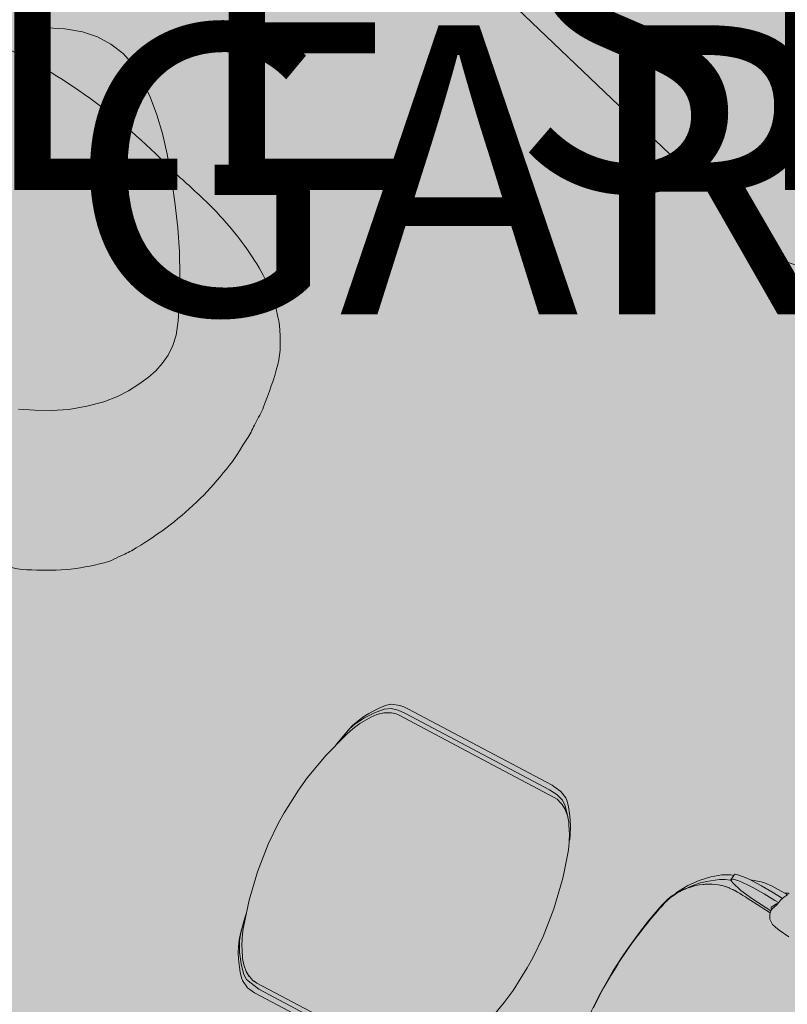
# Model space of a CAD drawing. Units: inches. Extents: x -466983 to 1020, y 324 to 318697.
# Tile 16 of 97: x 782.02 to 797.94, y 452.46 to 472.89. Entities that reach past the tile are written whole.
import ezdxf

# ---------------------------------------------------------------- set-up
doc = ezdxf.new("R2010")
doc.units = ezdxf.units.IN
doc.header["$MEASUREMENT"] = 0
for name, color, linetype, lineweight in [('A-ANNO-DIMS', 2, 'Continuous', 18), ('A-FLOR-PATT', 252, 'Continuous', 13), ('A-FURN', 8, 'Continuous', 18)]:
    doc.layers.add(name, color=color, linetype=linetype, lineweight=lineweight)
doc.layers.add('K-Hatch', color=7, linetype='Continuous')
doc.styles.get("Standard").update_dxf_attribs({"font": 'arial.ttf'})
doc.dimstyles.get("Standard").update_dxf_attribs({"dimtxt": 6, "dimasz": 4, "dimexe": 3, "dimexo": 3, "dimgap": 0.09, "dimtad": 0, "dimtih": 1, "dimtoh": 1, "dimdec": 1, "dimzin": 0, "dimdsep": 46, "dimlunit": 3, "dimtxsty": 'Standard', "dimcen": 0.09, "dimadec": 0, "dimazin": 0, "dimtfac": 1, "dimtdec": 1, "dimtofl": 0, "dimtmove": 0, "dimatfit": 3, "dimfxl": 1, "dimtolj": 1, "dimtzin": 0, "dimarcsym": 0})

# ---------------------------------------------------------------- blocks, each defined once
blk = doc.blocks.new('CBV_08')
at = {"layer": 'K-Hatch'}
h = blk.add_hatch(color=256, dxfattribs=at)
h.dxf.hatch_style = 1
h.set_gradient(color1=(254, 240, 205), color2=(128, 128, 128), name='INVSPHERICAL')
edge = h.paths.add_edge_path()
edge.add_line((-64.8, 606.5), (-20.8, 613.5))
edge.add_line((-20.8, 613.5), (24.3, 618.7))
edge.add_line((24.3, 618.7), (72.9, 622.4))
edge.add_line((72.9, 622.4), (121.2, 624.4))
edge.add_line((121.2, 624.4), (138, 624.4))
edge.add_spline(control_points=[(138, 624.4), (115.4, 642), (92.5, 659.2), (69.5, 676.1)], knot_values=[4, 4, 4, 4, 4.295361, 4.295361, 4.295361, 4.295361], degree=3, periodic=0)
edge.add_spline(control_points=[(69.5, 676.1), (30.7, 704.6), (-11, 728.2), (-55.3, 747.2)], knot_values=[3, 3, 3, 3, 4, 4, 4, 4], degree=3, periodic=0)
edge.add_spline(control_points=[(-55.3, 747.2), (-74.8, 755.6), (-96, 763.3), (-117, 767)], knot_values=[2, 2, 2, 2, 3, 3, 3, 3], degree=3, periodic=0)
edge.add_spline(control_points=[(-117, 767), (-129.2, 769.1), (-142.6, 773.4), (-154.9, 773.6)], knot_values=[1, 1, 1, 1, 2, 2, 2, 2], degree=3, periodic=0)
edge.add_spline(control_points=[(-154.9, 773.6), (-167.5, 773.8), (-180, 774.1), (-192.6, 774.3)], knot_values=[0, 0, 0, 0, 1, 1, 1, 1], degree=3, periodic=0)
edge.add_spline(control_points=[(-192.6, 774.3), (-216.8, 770.8), (-242.2, 768.1), (-264.6, 757.4)], knot_values=[36, 36, 36, 36, 37, 37, 37, 37], degree=3, periodic=0)
edge.add_spline(control_points=[(-264.6, 757.4), (-290.4, 745.1), (-313.9, 731.3), (-338.2, 716.3)], knot_values=[35, 35, 35, 35, 36, 36, 36, 36], degree=3, periodic=0)
edge.add_spline(control_points=[(-338.2, 716.3), (-348, 710.3), (-356.8, 702.3), (-365.9, 695.4)], knot_values=[34, 34, 34, 34, 35, 35, 35, 35], degree=3, periodic=0)
edge.add_spline(control_points=[(-365.9, 695.4), (-373.7, 689.5), (-381.9, 684), (-389, 677.3)], knot_values=[33, 33, 33, 33, 34, 34, 34, 34], degree=3, periodic=0)
edge.add_spline(control_points=[(-389, 677.3), (-406.7, 660.6), (-425.2, 644.6), (-441, 625.9)], knot_values=[32, 32, 32, 32, 33, 33, 33, 33], degree=3, periodic=0)
edge.add_spline(control_points=[(-441, 625.9), (-457.4, 606.6), (-473.1, 588.1), (-486.9, 566.8)], knot_values=[31, 31, 31, 31, 32, 32, 32, 32], degree=3, periodic=0)
edge.add_spline(control_points=[(-486.9, 566.8), (-500.9, 545.3), (-513.6, 524.6), (-525.3, 501.8)], knot_values=[30, 30, 30, 30, 31, 31, 31, 31], degree=3, periodic=0)
edge.add_spline(control_points=[(-525.3, 501.8), (-537.3, 478.5), (-547, 455.6), (-556.5, 431.1)], knot_values=[29, 29, 29, 29, 30, 30, 30, 30], degree=3, periodic=0)
edge.add_spline(control_points=[(-556.5, 431.1), (-560.1, 422), (-562.6, 413.9), (-564.7, 404.4)], knot_values=[28, 28, 28, 28, 29, 29, 29, 29], degree=3, periodic=0)
edge.add_spline(control_points=[(-564.7, 404.4), (-567.4, 392.4), (-572.8, 378.6), (-573.3, 366.3)], knot_values=[27, 27, 27, 27, 28, 28, 28, 28], degree=3, periodic=0)
edge.add_spline(control_points=[(-573.3, 366.3), (-574.1, 341.5), (-575.3, 317.8), (-572.6, 293.2)], knot_values=[26, 26, 26, 26, 27, 27, 27, 27], degree=3, periodic=0)
edge.add_spline(control_points=[(-572.6, 293.2), (-569.8, 268.3), (-564.7, 244.8), (-559.2, 220.4)], knot_values=[25, 25, 25, 25, 26, 26, 26, 26], degree=3, periodic=0)
edge.add_spline(control_points=[(-559.2, 220.4), (-554.1, 197.5), (-542.3, 175), (-531.2, 154.5)], knot_values=[24, 24, 24, 24, 25, 25, 25, 25], degree=3, periodic=0)
edge.add_spline(control_points=[(-531.2, 154.5), (-519.4, 132.5), (-505, 113.3), (-490.3, 93.1)], knot_values=[23, 23, 23, 23, 24, 24, 24, 24], degree=3, periodic=0)
edge.add_spline(control_points=[(-490.3, 93.1), (-483.4, 83.5), (-474, 75.1), (-466, 66.4)], knot_values=[22, 22, 22, 22, 23, 23, 23, 23], degree=3, periodic=0)
edge.add_spline(control_points=[(-466, 66.4), (-459.7, 59.5), (-453.6, 52.4), (-446.7, 46)], knot_values=[21, 21, 21, 21, 22, 22, 22, 22], degree=3, periodic=0)
edge.add_spline(control_points=[(-446.7, 46), (-428.9, 29.8), (-411.7, 12.8), (-392.8, -2.2)], knot_values=[20, 20, 20, 20, 21, 21, 21, 21], degree=3, periodic=0)
edge.add_spline(control_points=[(-392.8, -2.2), (-354.9, -32.3), (-316.7, -63.5), (-274.7, -87.8)], knot_values=[19, 19, 19, 19, 20, 20, 20, 20], degree=3, periodic=0)
edge.add_spline(control_points=[(-274.7, -87.8), (-235, -110.9), (-195.1, -133.6), (-153.3, -152.9)], knot_values=[18.058389, 18.058389, 18.058389, 18.058389, 19, 19, 19, 19], degree=3, periodic=0)
edge.add_arc((49.9, -261.3), 230.3, 65.0387, 151.9024, ccw=False)
edge.add_arc((-129.3, -568), 584.8, 31.4853, 61.8022, ccw=False)
edge.add_spline(control_points=[(369.5, -262.5), (382.1, -256.3), (394.4, -248.9), (404.8, -240.3)], knot_values=[14, 14, 14, 14, 14.639139, 14.639139, 14.639139, 14.639139], degree=3, periodic=0)
edge.add_spline(control_points=[(404.8, -240.3), (441.3, -209.9), (479.6, -177), (505.1, -136.3)], knot_values=[13, 13, 13, 13, 14, 14, 14, 14], degree=3, periodic=0)
edge.add_spline(control_points=[(505.1, -136.3), (530.8, -95.3), (553.2, -52.4), (563.4, -4.8)], knot_values=[12, 12, 12, 12, 13, 13, 13, 13], degree=3, periodic=0)
edge.add_spline(control_points=[(563.4, -4.8), (565.9, 6.8), (569.9, 18.9), (570.9, 30.6)], knot_values=[11, 11, 11, 11, 12, 12, 12, 12], degree=3, periodic=0)
edge.add_spline(control_points=[(570.9, 30.6), (572, 44.6), (573.1, 58.6), (574.2, 72.5)], knot_values=[10, 10, 10, 10, 11, 11, 11, 11], degree=3, periodic=0)
edge.add_spline(control_points=[(574.2, 72.5), (575.1, 84.1), (571.6, 97.4), (570.3, 109)], knot_values=[9, 9, 9, 9, 10, 10, 10, 10], degree=3, periodic=0)
edge.add_spline(control_points=[(570.3, 109), (569.1, 120.8), (562.9, 133.2), (559.3, 144.5)], knot_values=[8, 8, 8, 8, 9, 9, 9, 9], degree=3, periodic=0)
edge.add_spline(control_points=[(559.3, 144.5), (552.8, 164.6), (542, 184.7), (531.4, 203)], knot_values=[7, 7, 7, 7, 8, 8, 8, 8], degree=3, periodic=0)
edge.add_spline(control_points=[(531.4, 203), (517.9, 226.2), (504.2, 248.2), (488.9, 270.1)], knot_values=[6, 6, 6, 6, 7, 7, 7, 7], degree=3, periodic=0)
edge.add_spline(control_points=[(488.9, 270.1), (469.9, 297.6), (449.2, 323.8), (427.6, 349.1)], knot_values=[5.661323, 5.661323, 5.661323, 5.661323, 6, 6, 6, 6], degree=3, periodic=0)
edge.add_line((427.6, 349.1), (424, 340.6))
edge.add_line((424, 340.6), (412.8, 320.4))
edge.add_line((412.8, 320.4), (399.8, 302.2))
edge.add_line((399.8, 302.2), (384.1, 283.9))
edge.add_line((384.1, 283.9), (364.2, 265.4))
edge.add_line((364.2, 265.4), (338.9, 246.4))
edge.add_line((338.9, 246.4), (310.9, 228.8))
edge.add_line((310.9, 228.8), (283, 214))
edge.add_line((283, 214), (254.8, 200.7))
edge.add_line((254.8, 200.7), (225.6, 187.8))
edge.add_line((225.6, 187.8), (191.9, 174.7))
edge.add_line((191.9, 174.7), (149.8, 160.6))
edge.add_line((149.8, 160.6), (105.2, 147.1))
edge.add_line((105.2, 147.1), (63.8, 135.5))
edge.add_line((63.8, 135.5), (25.5, 126.4))
edge.add_line((25.5, 126.4), (-10.1, 120.3))
edge.add_line((-10.1, 120.3), (-42.7, 117))
edge.add_line((-42.7, 117), (-72.3, 116.4))
edge.add_line((-72.3, 116.4), (-101, 119.4))
edge.add_line((-101, 119.4), (-131.2, 126.4))
edge.add_line((-131.2, 126.4), (-161, 137.6))
edge.add_line((-161, 137.6), (-188.5, 153.1))
edge.add_line((-188.5, 153.1), (-212.6, 173.8))
edge.add_line((-212.6, 173.8), (-232.4, 200.6))
edge.add_line((-232.4, 200.6), (-247.5, 230.4))
edge.add_line((-247.5, 230.4), (-258, 260.2))
edge.add_line((-258, 260.2), (-265.5, 290.4))
edge.add_line((-265.5, 290.4), (-271.7, 321.1))
edge.add_line((-271.7, 321.1), (-275.7, 353.5))
edge.add_line((-275.7, 353.5), (-276.1, 388.5))
edge.add_line((-276.1, 388.5), (-273.5, 421.6))
edge.add_line((-273.5, 421.6), (-268.6, 448.2))
edge.add_line((-268.6, 448.2), (-261.6, 470.9))
edge.add_line((-261.6, 470.9), (-253.2, 492.6))
edge.add_line((-253.2, 492.6), (-243.7, 512.2))
edge.add_line((-243.7, 512.2), (-233.7, 528.6))
edge.add_line((-233.7, 528.6), (-222.4, 543.2))
edge.add_line((-222.4, 543.2), (-208.8, 557))
edge.add_line((-208.8, 557), (-193, 569.1))
edge.add_line((-193, 569.1), (-174.9, 578.6))
edge.add_line((-174.9, 578.6), (-149, 587.3))
edge.add_line((-149, 587.3), (-109.9, 597.2))
edge.add_line((-109.9, 597.2), (-64.8, 606.5))
edge = h.paths.add_edge_path()
edge.add_spline(control_points=[(370.8, -764.2), (495.7, -715.3), (556.2, -553.3), (490.4, -435.8)], knot_values=[8, 8, 8, 8, 9, 9, 9, 9], degree=3, periodic=0)
edge.add_spline(control_points=[(490.4, -435.8), (456.6, -375.3), (415.1, -316.6), (369.5, -262.5)], knot_values=[7.311196, 7.311196, 7.311196, 7.311196, 8, 8, 8, 8], degree=3, periodic=0)
edge.add_spline(control_points=[(369.5, -262.5), (362.3, -266), (355, -269.1), (347.9, -271.7)], knot_values=[14.639139, 14.639139, 14.639139, 14.639139, 15, 15, 15, 15], degree=3, periodic=0)
edge.add_spline(control_points=[(347.9, -271.7), (326, -279.9), (303.4, -287.9), (279.6, -286.9)], knot_values=[15, 15, 15, 15, 16, 16, 16, 16], degree=3, periodic=0)
edge.add_spline(control_points=[(279.6, -286.9), (229.3, -284.8), (181, -274.1), (132.3, -261.7)], knot_values=[16, 16, 16, 16, 17, 17, 17, 17], degree=3, periodic=0)
edge.add_spline(control_points=[(132.3, -261.7), (36, -237.2), (-55, -196.9), (-145.5, -156.4)], knot_values=[17, 17, 17, 17, 18, 18, 18, 18], degree=3, periodic=0)
edge.add_spline(control_points=[(-145.5, -156.4), (-148.1, -155.2), (-150.7, -154.1), (-153.3, -152.9)], knot_values=[18, 18, 18, 18, 18.058389, 18.058389, 18.058389, 18.058389], degree=3, periodic=0)
edge.add_spline(control_points=[(-274.7, -87.8), (-235, -110.9), (-195.1, -133.6), (-153.3, -152.9)], knot_values=[18.058389, 18.058389, 18.058389, 18.058389, 19, 19, 19, 19], degree=3, periodic=0)
edge.add_spline(control_points=[(-153.3, -152.9), (-166, -171.6), (-175.5, -191.9), (-179.2, -212.7)], knot_values=[4, 4, 4, 4, 4.452929, 4.452929, 4.452929, 4.452929], degree=3, periodic=0)
edge.add_spline(control_points=[(-179.2, -212.7), (-197.4, -316.3), (-177.2, -425), (-133.8, -520.2)], knot_values=[3, 3, 3, 3, 4, 4, 4, 4], degree=3, periodic=0)
edge.add_spline(control_points=[(-133.8, -520.2), (-113.8, -564.2), (-89.7, -609.8), (-55.6, -644.7)], knot_values=[2, 2, 2, 2, 3, 3, 3, 3], degree=3, periodic=0)
edge.add_spline(control_points=[(-55.6, -644.7), (-21, -680), (24.1, -705.5), (69.8, -723.3)], knot_values=[1, 1, 1, 1, 2, 2, 2, 2], degree=3, periodic=0)
edge.add_spline(control_points=[(69.8, -723.3), (165.7, -760.7), (268.3, -790.7), (370.8, -764.2)], knot_values=[0, 0, 0, 0, 1, 1, 1, 1], degree=3, periodic=0)
h = blk.add_hatch(color=256, dxfattribs=at)
h.dxf.hatch_style = 1
h.set_gradient(color1=(237, 238, 153), color2=(128, 128, 128), name='INVSPHERICAL')
h.paths.add_polyline_path([(138, 624.4), (121.2, 624.4), (72.9, 622.4), (24.3, 618.7), (-20.8, 613.5), (-64.8, 606.5), (-109.9, 597.2), (-149, 587.3), (-174.9, 578.6), (-193, 569.1), (-208.8, 557), (-222.4, 543.2), (-233.7, 528.6), (-243.7, 512.2), (-253.2, 492.6), (-261.6, 470.9), (-268.6, 448.2), (-273.5, 421.6), (-276.1, 388.5), (-275.7, 353.5), (-271.7, 321.1), (-265.5, 290.4), (-258, 260.2), (-247.5, 230.4), (-232.4, 200.6), (-212.6, 173.8), (-188.5, 153.1), (-161, 137.6), (-131.2, 126.4), (-101, 119.4), (-72.3, 116.4), (-42.7, 117), (-10.1, 120.3), (25.5, 126.4), (63.8, 135.5), (105.2, 147.1), (149.8, 160.6), (191.9, 174.7), (225.6, 187.8), (254.8, 200.7), (283, 214), (310.9, 228.8), (338.9, 246.4), (364.2, 265.4), (384.1, 283.9), (399.8, 302.2), (412.8, 320.4), (424, 340.6), (427.6, 349.1, 0.092765)])
h.paths.add_polyline_path([(388.8, 558), (367.1, 577.3), (341.1, 593.1), (309.7, 604.8), (275.6, 613.2), (241.4, 619.1), (205.2, 622.8), (165.2, 624.5), (138, 624.4, -0.092765), (427.6, 349.1), (434.3, 364.7), (441.6, 390.8), (443.8, 416.8), (441.1, 445), (433.5, 477.6), (421.8, 509.5), (406.9, 535.9)])
edge = h.paths.add_edge_path()
edge.add_arc((49.9, -261.3), 230.3, 65.0387, 151.9024)
edge.add_spline(control_points=[(-153.3, -152.9), (-150.7, -154.1), (-148.1, -155.2), (-145.5, -156.4)], knot_values=[18, 18, 18, 18, 18.058389, 18.058389, 18.058389, 18.058389], degree=3, periodic=0)
edge.add_spline(control_points=[(-145.5, -156.4), (-55, -196.9), (36, -237.2), (132.3, -261.7)], knot_values=[17, 17, 17, 17, 18, 18, 18, 18], degree=3, periodic=0)
edge.add_spline(control_points=[(132.3, -261.7), (181, -274.1), (229.3, -284.8), (279.6, -286.9)], knot_values=[16, 16, 16, 16, 17, 17, 17, 17], degree=3, periodic=0)
edge.add_spline(control_points=[(279.6, -286.9), (303.4, -287.9), (326, -279.9), (347.9, -271.7)], knot_values=[15, 15, 15, 15, 16, 16, 16, 16], degree=3, periodic=0)
edge.add_spline(control_points=[(347.9, -271.7), (355, -269.1), (362.3, -266), (369.5, -262.5)], knot_values=[14.639139, 14.639139, 14.639139, 14.639139, 15, 15, 15, 15], degree=3, periodic=0)
edge.add_arc((-129.3, -568), 584.8, 31.4853, 61.8022)
edge = h.paths.add_edge_path()
edge.add_spline(control_points=[(490.4, -435.8), (456.6, -375.3), (415.1, -316.6), (369.5, -262.5)], knot_values=[7.311196, 7.311196, 7.311196, 7.311196, 8, 8, 8, 8], degree=3, periodic=0)
edge.add_spline(control_points=[(369.5, -262.5), (362.3, -266), (355, -269.1), (347.9, -271.7)], knot_values=[14.639139, 14.639139, 14.639139, 14.639139, 15, 15, 15, 15], degree=3, periodic=0)
edge.add_spline(control_points=[(347.9, -271.7), (326, -279.9), (303.4, -287.9), (279.6, -286.9)], knot_values=[15, 15, 15, 15, 16, 16, 16, 16], degree=3, periodic=0)
edge.add_spline(control_points=[(279.6, -286.9), (229.3, -284.8), (181, -274.1), (132.3, -261.7)], knot_values=[16, 16, 16, 16, 17, 17, 17, 17], degree=3, periodic=0)
edge.add_spline(control_points=[(132.3, -261.7), (36, -237.2), (-55, -196.9), (-145.5, -156.4)], knot_values=[17, 17, 17, 17, 18, 18, 18, 18], degree=3, periodic=0)
edge.add_spline(control_points=[(-145.5, -156.4), (-148.1, -155.2), (-150.7, -154.1), (-153.3, -152.9)], knot_values=[18, 18, 18, 18, 18.058389, 18.058389, 18.058389, 18.058389], degree=3, periodic=0)
edge.add_spline(control_points=[(-274.7, -87.8), (-235, -110.9), (-195.1, -133.6), (-153.3, -152.9)], knot_values=[18.058389, 18.058389, 18.058389, 18.058389, 19, 19, 19, 19], degree=3, periodic=0)
edge.add_spline(control_points=[(-153.3, -152.9), (-166, -171.6), (-175.5, -191.9), (-179.2, -212.7)], knot_values=[4, 4, 4, 4, 4.452929, 4.452929, 4.452929, 4.452929], degree=3, periodic=0)
edge.add_spline(control_points=[(-179.2, -212.7), (-197.4, -316.3), (-177.2, -425), (-133.8, -520.2)], knot_values=[3, 3, 3, 3, 4, 4, 4, 4], degree=3, periodic=0)
edge.add_spline(control_points=[(-133.8, -520.2), (-113.8, -564.2), (-89.7, -609.8), (-55.6, -644.7)], knot_values=[2, 2, 2, 2, 3, 3, 3, 3], degree=3, periodic=0)
edge.add_spline(control_points=[(-55.6, -644.7), (-21, -680), (24.1, -705.5), (69.8, -723.3)], knot_values=[1, 1, 1, 1, 2, 2, 2, 2], degree=3, periodic=0)
edge.add_spline(control_points=[(69.8, -723.3), (165.7, -760.7), (268.3, -790.7), (370.8, -764.2)], knot_values=[0, 0, 0, 0, 1, 1, 1, 1], degree=3, periodic=0)
edge.add_spline(control_points=[(370.8, -764.2), (495.7, -715.3), (556.2, -553.3), (490.4, -435.8)], knot_values=[8, 8, 8, 8, 9, 9, 9, 9], degree=3, periodic=0)
for points in [[(24.3, 618.7), (-20.8, 613.5)], [(72.9, 622.4), (24.3, 618.7)], [(121.2, 624.4), (72.9, 622.4)], [(121.2, 624.4), (72.9, 622.4)], [(165.2, 624.5), (121.2, 624.4)], [(205.2, 622.8), (165.2, 624.5)], [(241.4, 619.1), (205.2, 622.8)], [(275.6, 613.2), (241.4, 619.1)], [(-109.9, 597.2), (-149, 587.3)], [(-64.8, 606.5), (-109.9, 597.2)], [(-20.8, 613.5), (-64.8, 606.5)], [(309.7, 604.8), (275.6, 613.2)], [(341.1, 593.1), (309.7, 604.8)], [(-174.9, 578.6), (-193, 569.1)], [(-149, 587.3), (-174.9, 578.6)], [(367.1, 577.3), (341.1, 593.1)], [(388.8, 558), (367.1, 577.3)], [(-193, 569.1), (-208.8, 557)], [(-222.4, 543.2), (-233.7, 528.6)], [(-208.8, 557), (-222.4, 543.2)], [(406.9, 535.9), (388.8, 558)], [(-233.7, 528.6), (-243.7, 512.2)], [(421.8, 509.5), (406.9, 535.9)], [(-243.7, 512.2), (-253.2, 492.6)], [(433.5, 477.6), (421.8, 509.5)], [(-253.2, 492.6), (-261.6, 470.9)], [(-261.6, 470.9), (-268.6, 448.2)], [(441.1, 445), (433.5, 477.6)], [(-268.6, 448.2), (-273.5, 421.6)], [(443.8, 416.8), (441.1, 445)], [(-273.5, 421.6), (-276.1, 388.5)], [(441.6, 390.8), (443.8, 416.8)], [(-276.1, 388.5), (-275.7, 353.5)], [(-275.7, 353.5), (-271.7, 321.1)], [(-271.7, 321.1), (-265.5, 290.4)], [(-265.5, 290.4), (-258, 260.2)]]:
    blk.add_lwpolyline(points)
at = {"ltscale": 150}
blk.add_arc((-452.8, -286.9), 1086.1, 35.8442, 57.0436, dxfattribs=at)
for points, knots in [([(427.6, 349.1), (449.2, 323.8), (469.9, 297.6), (488.9, 270.1), (504.2, 248.2), (517.9, 226.2), (531.4, 203), (542, 184.7), (552.8, 164.6), (559.3, 144.5), (562.9, 133.2), (569.1, 120.8), (570.3, 109), (571.6, 97.4), (575.1, 84.1), (574.2, 72.5), (573.1, 58.6), (572, 44.6), (570.9, 30.6), (569.9, 18.9), (565.9, 6.8), (563.4, -4.8), (553.2, -52.4), (530.8, -95.3), (505.1, -136.3), (479.6, -177), (441.3, -209.9), (404.8, -240.3), (388.6, -253.7), (367.6, -264.4), (347.9, -271.7), (326, -279.9), (303.4, -287.9), (279.6, -286.9), (229.3, -284.8), (181, -274.1), (132.3, -261.7), (36, -237.2), (-55, -196.9), (-145.5, -156.4), (-190.2, -136.4), (-232.5, -112.4), (-274.7, -87.8), (-316.7, -63.5), (-354.9, -32.3), (-392.8, -2.2), (-411.7, 12.8), (-428.9, 29.8), (-446.7, 46), (-453.6, 52.4), (-459.7, 59.5), (-466, 66.4), (-474, 75.1), (-483.4, 83.5), (-490.3, 93.1), (-505, 113.3), (-519.4, 132.5), (-531.2, 154.5), (-542.3, 175), (-554.1, 197.5), (-559.2, 220.4), (-564.7, 244.8), (-569.8, 268.3), (-572.6, 293.2), (-575.3, 317.8), (-574.1, 341.5), (-573.3, 366.3), (-572.8, 378.6), (-567.4, 392.4), (-564.7, 404.4), (-562.6, 413.9), (-560.1, 422), (-556.5, 431.1), (-547, 455.6), (-537.3, 478.5), (-525.3, 501.8), (-513.6, 524.6), (-500.9, 545.3), (-486.9, 566.8), (-473.1, 588.1), (-457.4, 606.6), (-441, 625.9), (-425.2, 644.6), (-406.7, 660.6), (-389, 677.3), (-381.9, 684), (-373.7, 689.5), (-365.9, 695.4), (-356.8, 702.3), (-348, 710.3), (-338.2, 716.3), (-313.9, 731.3), (-290.4, 745.1), (-264.6, 757.4), (-242.2, 768.1), (-216.8, 770.8), (-192.6, 774.3)], [5.661323, 5.661323, 5.661323, 5.661323, 6, 6, 6, 7, 7, 7, 8, 8, 8, 9, 9, 9, 10, 10, 10, 11, 11, 11, 12, 12, 12, 13, 13, 13, 14, 14, 14, 15, 15, 15, 16, 16, 16, 17, 17, 17, 18, 18, 18, 19, 19, 19, 20, 20, 20, 21, 21, 21, 22, 22, 22, 23, 23, 23, 24, 24, 24, 25, 25, 25, 26, 26, 26, 27, 27, 27, 28, 28, 28, 29, 29, 29, 30, 30, 30, 31, 31, 31, 32, 32, 32, 33, 33, 33, 34, 34, 34, 35, 35, 35, 36, 36, 36, 37, 37, 37, 37]), ([(-192.6, 774.3), (-180, 774.1), (-167.5, 773.8), (-154.9, 773.6), (-142.6, 773.4), (-129.2, 769.1), (-117, 767), (-96, 763.3), (-74.8, 755.6), (-55.3, 747.2), (-11, 728.2), (30.7, 704.6), (69.5, 676.1), (92.5, 659.2), (115.4, 642), (138, 624.4)], [0, 0, 0, 0, 1, 1, 1, 2, 2, 2, 3, 3, 3, 4, 4, 4, 4.295361, 4.295361, 4.295361, 4.295361])]:
    blk.add_open_spline(points, degree=3, knots=knots)
blk = doc.blocks.new('CBV_05')
at = {"layer": 'K-Hatch'}
h = blk.add_hatch(color=256, dxfattribs=at)
h.dxf.hatch_style = 1
h.paths.add_polyline_path([(614, 437), (1251.4, 62.5), (1198.3, -263.2), (564.8, -9.8), (344.4, -5.5), (343.7, -629.7, 0.159768), (369.9, -672.6), (1020.5, -1025.6, 0.317347), (1135.5, -1017.7), (1739.5, -492.7, 0.378101), (1761.2, -362.2), (1507.4, -70.4, -0.119239), (1492.6, -25.8), (1499.5, 665.1, 0.256804), (1446.2, 745.4), (822.7, 1028.7, 0.297137), (714, 1018.3), (625, 963.6), (549.5, 1037.1), (186.8, 587.5), (-1106.2, 397.7), (-1098.6, 311.5), (-1098.4, 310.2)])
h.paths.add_polyline_path([(344.4, -5.5), (-1216.9, 24.6), (-1212.3, 260), (-1718.1, 162.7, 0.51466), (-1765.1, 50), (-1478.1, -479.5, 0.244482), (-1398.8, -526.6), (323.6, -658.2, 0.453292), (343.1, -629.8, 0.006511), (343.7, -631.8)])
blk.add_lwpolyline([(1761.2, -362.2, -0.378101), (1739.5, -492.7), (1135.5, -1017.7, -0.317347), (1020.5, -1025.6), (369.9, -672.6, -0.159481), (343.2, -630.1, -0.449095), (323.6, -658.2), (-1398.8, -526.6, -0.244482), (-1478.1, -479.5), (-1765.1, 50, -0.51466), (-1718.1, 162.7), (-1212.3, 260), (-1211.5, 301.9), (-1098.4, 310.2), (-1106.2, 397.7), (186.8, 587.5), (549.5, 1037.1), (625, 963.6), (714, 1018.3, -0.297137), (822.7, 1028.7), (1446.2, 745.4, -0.256804), (1499.5, 665.1), (1492.6, -25.8, 0.119239), (1507.4, -70.4)], format="xyb", close=True)
blk.add_lwpolyline([(-1212.3, 260), (-1718.1, 162.7, 0.51466), (-1765.1, 50), (-1478.1, -479.5, 0.244482), (-1398.8, -526.6), (323.6, -658.2)], format="xyb")
blk = doc.blocks.new('CBV_11')
at = {"layer": 'K-Hatch'}
h = blk.add_hatch(color=256, dxfattribs=at)
h.dxf.hatch_style = 1
h.paths.add_polyline_path([(-178.4, 698.3), (-200.4, 717.9), (-207.1, 720), (-213, 721.7), (-231.8, 722.5), (-254.2, 721.5), (-275, 717.7), (-289.3, 712.5), (-316, 699.4), (-324.9, 694.8), (-295.8, 706.5), (-286.8, 709.3), (-277.1, 712.2), (-265.3, 715), (-258.1, 715.9), (-241.3, 718.1), (-228.8, 718), (-215.5, 715.7), (-208.8, 713.2), (-205.5, 711.6), (-203.9, 710.6), (-202.4, 709.7), (-195.4, 705.2), (-194.8, 704.5), (-190.4, 699.8), (-87.3, 570), (16.1, 440.3), (19.6, 435), (22.9, 426.4), (24.1, 422.9), (25.8, 412.3), (25.1, 398.9), (24.2, 394.5), (25.6, 399.8), (28.8, 418.8), (27.5, 432), (13.6, 457)])
h.paths.add_polyline_path([(-536, 213.1), (-639.3, 342.7), (-642.9, 348.1), (-646.2, 356.7), (-647.4, 360.2), (-649.1, 370.8), (-648.4, 384.2), (-645.7, 396.4), (-637.3, 419.1), (-631.8, 430), (-626.9, 438.8), (-622.1, 446.9), (-606.5, 469.3), (-631, 439.9), (-638.6, 427.4), (-646.5, 408.6), (-652.3, 388), (-655.6, 368.8), (-654.4, 355.7), (-649, 343.1), (-640.5, 330.7), (-448.6, 89.4), (-437.6, 77.7), (-424.8, 69.2), (-413.8, 65.9), (-392.4, 64.7), (-388.1, 65), (-394.5, 65), (-407.8, 67.4), (-417, 71.1), (-420.9, 73.4), (-427.9, 77.9), (-428.5, 78.6), (-432.9, 83.2)])
for points in [[(21.3, 463.1), (-173.2, 707.5), (-185, 718.7), (-200.1, 726), (-205.3, 726.9), (-216.4, 727.2), (-226.1, 726.9), (-241.2, 725.8), (-253.7, 723.9), (-264.9, 721.5), (-277.2, 717.9), (-288.3, 713.3), (-311.8, 701.8), (-324.9, 694.8), (-316, 699.4), (-289.3, 712.5), (-275, 717.7), (-254.2, 721.5), (-231.8, 722.5), (-213, 721.7), (-207.1, 720), (-200.4, 717.9), (-178.4, 698.3), (13.6, 457)], [(-87.3, 570), (-190.4, 699.8), (-194.8, 704.5), (-195.4, 705.2), (-202.4, 709.7), (-203.9, 710.6), (-208.8, 713.2), (-215.5, 715.7), (-228.8, 718), (-241.3, 718.1), (-258.1, 715.9), (-265.3, 715), (-277.1, 712.2), (-286.8, 709.3), (-295.8, 706.5), (-324.9, 694.8), (-347.4, 685.7), (-397.3, 660.4), (-444.8, 630.8), (-480.8, 604.2), (-497.4, 590.5), (-534.5, 556.2), (-554.4, 535.5), (-590.2, 492.6), (-603.5, 473.5), (-606.5, 469.3), (-622.1, 446.9), (-626.9, 438.8), (-631.8, 430), (-637.3, 419.1), (-645.7, 396.4), (-648.4, 384.2), (-649.1, 370.8), (-647.4, 360.2), (-646.2, 356.7), (-642.9, 348.1), (-639.3, 342.7), (-536, 213.1), (-432.9, 83.2), (-428.5, 78.6), (-427.9, 77.9), (-420.9, 73.4), (-417, 71.1), (-407.8, 67.4), (-394.5, 65), (-388.1, 65), (-382, 64.9), (-376.6, 65.6), (-368.3, 66.6), (-367.7, 66.7), (-359.3, 67.5), (-346.5, 70.4), (-345.9, 70.6), (-336.1, 73.3), (-327.3, 76.2), (-282.4, 94.4), (-275.6, 97.1), (-225.7, 122.4), (-178.3, 151.9), (-142.2, 178.6), (-125.6, 192.2), (-88.5, 226.6), (-68.7, 247.3), (-32.9, 290.2)], [(-203.9, 710.6), (-205.5, 711.6), (-208.8, 713.2)], [(-346.5, 70.4), (-349.3, 69.2), (-356.8, 67), (-372.9, 63.3), (-385.5, 61.5), (-398.1, 60.5), (-410.3, 60.2), (-421.5, 60.6), (-428.5, 61.9), (-441.8, 68.9), (-453.7, 80.2), (-456.3, 83.2), (-648.2, 324.6), (-653.1, 331.3), (-657.2, 338.3), (-662.3, 353.4), (-662.3, 363.4), (-659.9, 375.1), (-656.8, 387), (-652.8, 399), (-648.1, 410.9), (-642.7, 422.1), (-636.8, 432.3), (-630.4, 441.2), (-607, 469.6), (-603.5, 473.5)], [(-606.5, 469.3), (-631, 439.9), (-638.6, 427.4), (-646.5, 408.6), (-652.3, 388), (-655.6, 368.8), (-654.4, 355.7), (-649, 343.1), (-640.5, 330.7), (-448.6, 89.4), (-437.6, 77.7), (-424.8, 69.2), (-413.8, 65.9), (-392.4, 64.7), (-388.1, 65)], [(-50.1, 67.5), (-23.5, 87.9), (-9.9, 97.6), (3.8, 107.1), (17.8, 116.4), (31.9, 125.3), (60.6, 142.4), (89.9, 158.3), (119.5, 173.3), (135, 179.9), (142.8, 182.8), (151, 184.8), (159.6, 185.9), (175.9, 186.9), (181, 186.7)], [(-28.5, 83.3), (-36.4, 77.2), (-38.8, 75.4), (-45.1, 70.6), (-49.7, 67), (-54.2, 63.4), (-56, 61.9), (-62.5, 56.6), (-75.5, 45.6), (-77.3, 44), (-77.4, 44)], [(-217.7, -216.8), (-218.7, -214.8), (-221.6, -206), (-223.5, -195.1), (-224.4, -170.3), (-223.2, -156.5), (-220.9, -142.4), (-219, -134.5), (-218.9, -134.4), (-218.9, -134.2), (-217.3, -125.9), (-215.2, -117.7), (-212.7, -109.9), (-212.1, -108.4), (-207.7, -98.2), (-203.6, -90.8), (-196.4, -80.6), (-191.3, -74), (-180.9, -61.1), (-170.2, -48.3), (-159.1, -35.9), (-159.1, -35.8), (-148, -23.5), (-124.9, 0.7), (-113, 12.4), (-100.8, 23.9), (-88.5, 35.1), (-75.9, 46.2), (-63.1, 57), (-50.1, 67.5)], [(-214.7, -118), (-214.6, -117.8), (-212.4, -111.4), (-210.9, -107.7), (-210.4, -106.5), (-210.1, -105.7), (-209.4, -104.2), (-209, -103.5), (-206, -97.3), (-205.1, -95.8), (-204.7, -95), (-203.9, -93.8), (-203.5, -93.2), (-202.6, -91.5), (-202, -90.5), (-200.3, -88.1), (-199.3, -86.6), (-198.2, -84.9), (-198, -84.7), (-197.9, -84.5), (-192.8, -77.9), (-190.9, -75.4), (-190.5, -74.9), (-189.8, -74), (-186.5, -69.8), (-173.8, -54.2), (-170.7, -50.6), (-169.2, -48.8), (-167, -46.3), (-160.8, -39.1), (-147.5, -24.2), (-147.4, -24.1), (-147.3, -24), (-146.9, -23.6), (-146.4, -23.1), (-134, -9.8), (-127, -2.7), (-124.7, -0.3), (-124.4, -0.1), (-124.2, 0.2), (-123.2, 1.2), (-120.2, 4.2), (-106.2, 17.9), (-102.9, 20.9), (-101.4, 22.4), (-98.9, 24.6), (-91.9, 31.1), (-77.7, 43.7), (-77.6, 43.8), (-77.4, 44)], [(-212.1, -108.4), (-213.8, -111.2), (-223, -134.4), (-228.6, -157.2), (-231.3, -180.4), (-231, -201.3), (-228.1, -217.6), (-225.8, -223.3), (-226.1, -223.6), (-227.6, -226.1), (-224.9, -232.9), (-218.3, -243.6), (-212.6, -251.5), (-209.6, -255.8), (-197.1, -271.4), (-182.6, -288.2), (-173.4, -298.4), (-166.3, -306.1)], [(-143.8, -278.1), (-149.7, -271.9), (-151.2, -270.2), (-153.6, -267.6), (-153.7, -267.6), (-158.2, -262.7), (-179.1, -240.4), (-181.9, -237.4), (-184, -235.2), (-185.8, -233.2), (-188.4, -230.4), (-188.8, -230), (-189.2, -229.5), (-191, -227.5), (-192.6, -225.7), (-192.9, -225.2), (-193.3, -224.8), (-194.6, -223.3), (-196.5, -221), (-197, -220.3), (-197.5, -219.7), (-198.5, -218.3), (-200, -216.4), (-200.2, -216.2), (-201.3, -214.6), (-201.4, -214.5), (-203.2, -212), (-203.8, -211.2), (-204.4, -210.2), (-205.3, -208.8), (-206.1, -207.6), (-206.2, -207.4), (-206.3, -207.3), (-206.4, -207), (-206.6, -206.8), (-207.1, -206), (-207.5, -205.3), (-207.5, -205.2), (-207.6, -205.1), (-207.6, -205), (-208.1, -204.2), (-208.2, -204), (-208.3, -203.8), (-208.4, -203.7), (-208.7, -203.2), (-209.4, -202), (-209.4, -201.9), (-209.6, -201.7), (-210.3, -200.2), (-211.3, -198.2), (-211.5, -197.7), (-212.6, -194.8), (-213.7, -191.8), (-214, -190.9), (-215.6, -185.2), (-217, -180.3), (-217, -180.3), (-217, -180.3), (-217.6, -177.7), (-218.5, -172.7), (-218.9, -170.6), (-219, -169.1), (-219.2, -168.2), (-219.2, -167.9), (-219.3, -167.8), (-219.3, -166.9), (-219.6, -165), (-219.8, -163.4), (-220.2, -156.1), (-220.2, -148.7), (-219.6, -142.8), (-219.6, -142.2), (-219.6, -142), (-219.6, -141.7), (-219.5, -141.2), (-218.5, -134), (-217.9, -130.8), (-217.7, -129.5), (-217.7, -129.3), (-217.5, -128.7), (-217.5, -128.6), (-217.4, -128.4), (-217, -126.3), (-215, -118.8), (-214.9, -118.6), (-214.9, -118.5), (-214.7, -118), (-214.9, -118.5)], [(-225.8, -223.3), (-218.8, -216.5), (-217.7, -216.8), (-213.1, -218.1), (-195.7, -231.2), (-175.3, -250.4), (-147.2, -280.1)], [(-159.9, -297.1), (-165.4, -291.2), (-181.5, -273.1), (-197.1, -254.2), (-203.8, -245.5), (-213.9, -230.9), (-219, -220.9), (-218.8, -216.5)], [(-212.6, -251.5), (-211.9, -253), (-204.6, -272.1), (-201.7, -277.7), (-192.5, -291.1), (-180.6, -305.8), (-175.6, -311.7), (-173.4, -314.3), (-171.3, -316.5)], [(-92.5, -304.3), (-108.7, -288.6), (-115.6, -282.9), (-121.5, -278.5), (-131.9, -275.3), (-141.2, -276.5), (-143.8, -278.1), (-147.2, -280.1), (-148.4, -280.8), (-149.5, -281.9), (-150.1, -282.4), (-156.3, -292.9), (-159.1, -296.2), (-158.4, -292.9), (-155.5, -285.3), (-153.9, -281.9), (-151.3, -281.2), (-149.5, -281.9)], [(-171.3, -316.5), (-167.5, -308.1), (-166.3, -306.1), (-163.8, -301.8), (-160.2, -297.5), (-159.9, -297.1), (-159.1, -296.2)], [(-175.6, -311.7), (-175.4, -312.6), (-174, -317.8), (-172.7, -319.6)]]:
    blk.add_lwpolyline(points)
blk = doc.blocks.new('Garden Sofa')
at = {"xscale": -0.0109740885734132, "yscale": 0.0109740885734132, "zscale": 0.0109740885734132}
for name, p, rotation in [('CBV_05', (2464.355, 846.083), 311.9356943688126), ('CBV_08', (2451.373, 829.781), 280.5267845499334), ('CBV_11', (2467.574, 814.959), 100.5267845499335)]:
    blk.add_blockref(name, p, dxfattribs=dict(at, rotation=rotation))
blk = doc.blocks.new('*D93')
at = {"layer": 'A-ANNO-DIMS', "color": 0, "lineweight": -2, "transparency": 16777216}
for p, q in [((808.966, 500.777), (818.266, 500.777)), ((815.266, 496.777), (815.266, 472.969)), ((815.266, 442.777), (815.266, 466.584)), ((808.966, 438.777), (818.266, 438.777))]:
    blk.add_line(p, q, dxfattribs=at)
at = {"layer": 'A-ANNO-DIMS', "color": 0, "transparency": 16777216}
for points in [[(814.599, 496.777), (815.933, 496.777), (815.266, 500.777)], [(814.599, 442.777), (815.933, 442.777), (815.266, 438.777)]]:
    blk.add_solid(points, dxfattribs=at)
at = {"layer": 'Defpoints', "color": 0, "transparency": 16777216}
for p in [(805.966, 500.777), (815.266, 500.777), (805.966, 438.777)]:
    blk.add_point(p, dxfattribs=at)
at = {"layer": 'A-ANNO-DIMS', "color": 0, "transparency": 16777216, "insert": (815.266, 469.777), "char_height": 6, "attachment_point": 5}
blk.add_mtext('\\A1;GARDEN SEAT 62', dxfattribs=at)
blk = doc.blocks.new('*D97')
at = {"layer": 'A-ANNO-DIMS', "color": 0, "lineweight": -2, "transparency": 16777216}
for p, q in [((823.929, 568.441), (802.329, 568.441)), ((805.329, 564.441), (805.329, 499.545)), ((805.329, 428.441), (805.329, 493.337)), ((823.929, 424.441), (802.329, 424.441))]:
    blk.add_line(p, q, dxfattribs=at)
at = {"layer": 'A-ANNO-DIMS', "color": 0, "transparency": 16777216}
for points in [[(804.662, 564.441), (805.996, 564.441), (805.329, 568.441)], [(804.662, 428.441), (805.996, 428.441), (805.329, 424.441)]]:
    blk.add_solid(points, dxfattribs=at)
at = {"layer": 'Defpoints', "color": 0, "transparency": 16777216}
for p in [(826.929, 568.441), (805.329, 424.441), (826.929, 424.441)]:
    blk.add_point(p, dxfattribs=at)
at = {"layer": 'A-ANNO-DIMS', "color": 0, "transparency": 16777216, "insert": (805.329, 496.441), "char_height": 6, "attachment_point": 5}
blk.add_mtext('\\A1;BIKE 144', dxfattribs=at)
blk = doc.blocks.new('*D113')
at = {"layer": 'A-ANNO-DIMS', "color": 0, "lineweight": -2, "transparency": 16777216}
for p, q in [((704.71, 504.652), (709.525, 509.413)), ((710.204, 504.46), (736.319, 478.049)), ((736.45, 472.553), (741.265, 477.314)), ((739.132, 475.204), (741.944, 472.36)), ((741.944, 472.36), (745.944, 472.36))]:
    blk.add_line(p, q, dxfattribs=at)
at = {"layer": 'A-ANNO-DIMS', "color": 0, "transparency": 16777216}
for points in [[(710.678, 504.928), (709.73, 503.991), (707.392, 507.304)], [(736.794, 478.517), (735.845, 477.58), (739.132, 475.204)]]:
    blk.add_solid(points, dxfattribs=at)
at = {"layer": 'Defpoints', "color": 0, "transparency": 16777216}
for p in [(702.577, 502.543), (739.132, 475.204), (734.317, 470.443)]:
    blk.add_point(p, dxfattribs=at)
at = {"layer": 'A-ANNO-DIMS', "color": 0, "transparency": 16777216, "insert": (783.502, 472.36), "char_height": 6, "attachment_point": 5}
blk.add_mtext('\\A1;TEA TABLE SET 45', dxfattribs=at)

msp = doc.modelspace()

# ---------------------------------------------------------------- hatches: boundary and pattern name
at = {"layer": 'A-FLOR-PATT', "transparency": 33554661}
h = msp.add_hatch(color=256, dxfattribs=at)
h.dxf.hatch_style = 1
h.set_gradient(color1=(19, 155, 72), color2=(0, 107, 0), name='CYLINDER')
h.paths.add_polyline_path([(813.806, 503.938), (730.806, 503.938), (730.806, 424.938), (612.806, 424.938), (612.806, 415.938), (442.806, 415.938), (442.806, 368.938), (813.806, 368.938)])
h.paths.add_polyline_path([(771.796, 407.07), (783.796, 407.07), (783.796, 371.07), (771.796, 371.07)], flags=16)
h.paths.add_polyline_path([(755.796, 407.07), (755.796, 371.07), (743.796, 371.07), (743.796, 407.07)], flags=16)
h.paths.add_polyline_path([(769.796, 404.07), (769.796, 374.07), (757.796, 374.07), (757.796, 404.07)], flags=16)
h.paths.add_polyline_path([(785.796, 404.07), (797.796, 404.07), (797.796, 374.07), (785.796, 374.07)], flags=16)
h.paths.add_polyline_path([(741.796, 404.07), (741.796, 374.07), (729.796, 374.07), (729.796, 404.07)], flags=16)
h.paths.add_polyline_path([(799.796, 407.07), (811.796, 407.07), (811.796, 371.07), (799.796, 371.07)], flags=16)
h.paths.add_polyline_path([(727.796, 407.07), (727.796, 371.07), (715.796, 371.07), (715.796, 407.07)], flags=16)
h.paths.add_polyline_path([(713.796, 404.07), (713.796, 374.07), (701.796, 374.07), (701.796, 404.07)], flags=16)
h.paths.add_polyline_path([(699.796, 407.07), (699.796, 371.07), (687.796, 371.07), (687.796, 407.07)], flags=16)
h.paths.add_polyline_path([(685.796, 404.07), (685.796, 374.07), (673.796, 374.07), (673.796, 404.07)], flags=16)
h.paths.add_polyline_path([(671.796, 407.07), (671.796, 371.07), (659.796, 371.07), (659.796, 407.07)], flags=16)
h.paths.add_polyline_path([(657.796, 404.07), (657.796, 374.07), (645.796, 374.07), (645.796, 404.07)], flags=16)
h.paths.add_polyline_path([(643.796, 407.07), (643.796, 371.07), (631.796, 371.07), (631.796, 407.07)], flags=16)
h.paths.add_polyline_path([(629.796, 404.07), (629.796, 374.07), (617.796, 374.07), (617.796, 404.07)], flags=16)
h.paths.add_polyline_path([(615.796, 407.07), (615.796, 371.07), (603.796, 371.07), (603.796, 407.07)], flags=16)
h.paths.add_polyline_path([(601.796, 404.07), (601.796, 374.07), (589.796, 374.07), (589.796, 404.07)], flags=16)
at = {"layer": 'A-FLOR-PATT'}
h = msp.add_hatch(dxfattribs=at)
h.set_pattern_fill('GRASS', color=256, scale=6)
h.set_pattern_definition([(90, (-1212.4137, -290.035), (-4.242641, 4.242641), [1.125, -7.360281]), (45, (-1212.4137, -290.035), (-4.24264, 4.24264), [1.125, -4.875]), (135, (-1212.4137, -290.035), (-4.24264, -4.24264), [1.125, -4.875])])
h.paths.add_polyline_path([(813.806, 503.938), (730.806, 503.938), (730.806, 424.938), (612.806, 424.938), (612.806, 415.938), (442.806, 415.938), (442.806, 368.938), (813.806, 368.938)])
h.paths.add_polyline_path([(589.796, 404.07), (601.796, 404.07), (601.796, 374.07), (589.796, 374.07)], flags=16)
h.paths.add_polyline_path([(603.796, 407.07), (615.796, 407.07), (615.796, 371.07), (603.796, 371.07)], flags=16)
h.paths.add_polyline_path([(617.796, 404.07), (629.796, 404.07), (629.796, 374.07), (617.796, 374.07)], flags=16)
h.paths.add_polyline_path([(631.796, 407.07), (643.796, 407.07), (643.796, 371.07), (631.796, 371.07)], flags=16)
h.paths.add_polyline_path([(645.796, 404.07), (657.796, 404.07), (657.796, 374.07), (645.796, 374.07)], flags=16)
h.paths.add_polyline_path([(659.796, 407.07), (671.796, 407.07), (671.796, 371.07), (659.796, 371.07)], flags=16)
h.paths.add_polyline_path([(673.796, 404.07), (685.796, 404.07), (685.796, 374.07), (673.796, 374.07)], flags=16)
h.paths.add_polyline_path([(687.796, 407.07), (699.796, 407.07), (699.796, 371.07), (687.796, 371.07)], flags=16)
h.paths.add_polyline_path([(701.796, 404.07), (713.796, 404.07), (713.796, 374.07), (701.796, 374.07)], flags=16)
h.paths.add_polyline_path([(715.796, 407.07), (727.796, 407.07), (727.796, 371.07), (715.796, 371.07)], flags=16)
h.paths.add_polyline_path([(729.796, 404.07), (741.796, 404.07), (741.796, 374.07), (729.796, 374.07)], flags=16)
h.paths.add_polyline_path([(743.796, 407.07), (755.796, 407.07), (755.796, 371.07), (743.796, 371.07)], flags=16)
h.paths.add_polyline_path([(757.796, 404.07), (769.796, 404.07), (769.796, 374.07), (757.796, 374.07)], flags=16)
h.paths.add_polyline_path([(771.796, 407.07), (783.796, 407.07), (783.796, 371.07), (771.796, 371.07)], flags=16)
h.paths.add_polyline_path([(785.796, 404.07), (797.796, 404.07), (797.796, 374.07), (785.796, 374.07)], flags=16)
h.paths.add_polyline_path([(799.796, 407.07), (811.796, 407.07), (811.796, 371.07), (799.796, 371.07)], flags=16)

# ---------------------------------------------------------------- block references
at = {"layer": 'A-FURN'}
msp.add_blockref('Garden Sofa', (-1672.7, -362.711), dxfattribs=at)

# ---------------------------------------------------------------- dimensions: what is measured, and where the dimension line sits
at = {"layer": 'A-ANNO-DIMS'}
for base, p1, p2, angle, text, picture, middle in [((805.329, 424.441), (826.929, 568.441), (826.929, 424.441), 270, 'BIKE <>', '*D97', (805.329, 496.441)), ((739.132, 475.204), (702.577, 502.543), (734.317, 470.443), 314.6775, 'TEA TABLE SET <>', '*D113', (783.502, 472.36)), ((815.266, 500.777), (805.966, 438.777), (805.966, 500.777), 90, 'GARDEN SEAT <>', '*D93', (815.266, 469.777))]:
    dim = msp.add_linear_dim(base=base, p1=p1, p2=p2, angle=angle, text=text, dimstyle='Standard', override={"dimdec": 0, "dimlfac": 1, "dimrnd": 0, "dimzin": 0, "dimdsep": 46, "dimlunit": 2}, dxfattribs=at)
    dim.commit()
    dim.dimension.update_dxf_attribs({"geometry": picture, "text_midpoint": middle})

doc.saveas('drawing.dxf')
